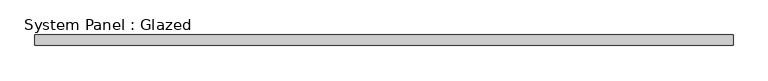
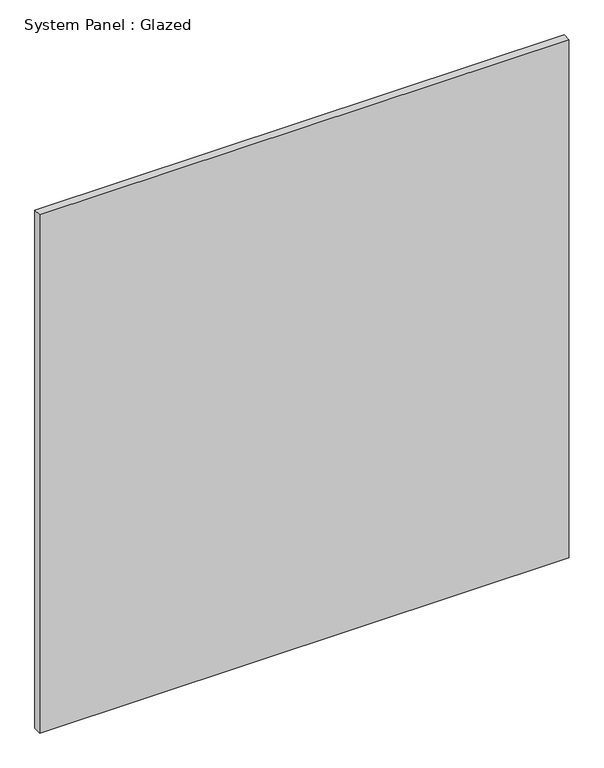
"""IFC4 building model written with IfcOpenShell, lengths in millimetres: plate geometry, System Panel : Glazed."""

from ifc_helpers import new_model, si_unit, origin, origin_with_axes, place, context, project, spatial, polyline, outline, extrude, source, transform, mapped, element, save


def system_panel_glazed_a1eab1ce(model_context):
    return source(origin(), model_context, "Body", "SweptSolid", [
        extrude(outline(polyline([(838.2, 19.05), (-838.2, 19.05), (-838.2, 44.45), (838.2, 44.45), (838.2, 19.05)])), origin_with_axes(), (0.0, 0.0, 1.0), 1735.2405875),
    ])


if __name__ == "__main__":
    model = new_model("IFC4")
    model_context = context("Model", 3, world=origin())
    ifc_project = project(units=[si_unit("LENGTHUNIT", "METRE", prefix="MILLI")], contexts=[model_context])
    site = spatial("IfcSite", under=ifc_project)
    building = spatial("IfcBuilding", under=site)
    placement = place(None, origin())
    system_panel_glazed_shape = system_panel_glazed_a1eab1ce(model_context)
    element("IfcPlate", 1, ObjectType="System Panel : Glazed", at=placement, inside=building, context=model_context, shape_type="MappedRepresentation", body=[
        mapped(system_panel_glazed_shape, transform((0.0, 0.0, 0.0), x_axis=(1.0, 0.0, 0.0), y_axis=(0.0, 1.0, 0.0), z_axis=(0.0, 0.0, 1.0))),
    ])
    save(model, "model.ifc")

# Revit data of these elements
# Type "System Panel : Glazed"
#   Construction Type Id = "GSP4R"
#   Analytic Construction = "1/8 in Pilkington single glazing"
#   Visual Light Transmittance = 0.9
#   Solar Heat Gain Coefficient = 0.86
#   Heat Transfer Coefficient (U) = 1.18115 BTU/(h·ft²·°F)
# Element 1 (IfcPlate, "System Panel : Glazed")
#   Materials on its faces: "Glass"
# Materials
#   "Glass": class "Glass", colour RGB 0 128 192, transparency 0.75, Description = "Soda Lime Glass", Cost = 0
